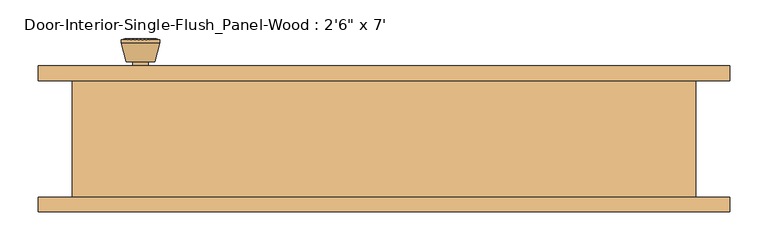
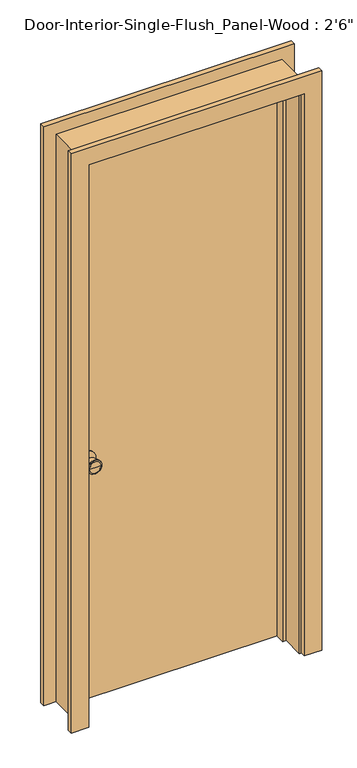
"""IFC4 building model written with IfcOpenShell, lengths in millimetres: door geometry."""

from ifc_helpers import new_model, si_unit, point, frame, frame_2d, origin, origin_with_axes, place, context, project, spatial, polyline, circle_curve, trimmed, segment, composite_curve, outline, extrude, faceted_brep, source, transform, mapped, element, save
from ifc_brep_helpers import plane_surface, cylinder_surface, revolved_surface, advanced_brep


def door_2b62d641(model_context):
    return source(origin(), model_context, "Body", "SolidModel", [
        advanced_brep(
        [(-317.5, 32.1, 914.4), (-307.5, 32.1, 914.4), (-327.5, 32.1, 914.4), (-297.0241324, -16.9, 914.4), (-317.5, -16.9, 914.4), (-337.9758676, -16.9, 914.4), (-292.5, -15.0721319, 914.4), (-342.5, -15.0721319, 914.4), (-292.5, -11.6084537, 914.4), (-342.5, -11.6084537, 914.4), (-298.863764, 13.1, 914.4), (-336.136236, 13.1, 914.4), (-307.5, 13.1, 914.4), (-327.5, 13.1, 914.4)],
        [
            (0, 1),
            (1, 2, circle_curve(frame((-317.5, 32.1, 914.4), z_axis=(0.0, 1.0, 0.0), x_axis=(-1.0, 0.0, 0.0)), 10.0)),
            (2, 0),
            (2, 1, circle_curve(frame((-317.5, 32.1, 914.4), z_axis=(0.0, 1.0, 0.0), x_axis=(-1.0, 0.0, 0.0)), 10.0)),
            (3, 4),
            (4, 5),
            (5, 3, circle_curve(frame((-317.5, -16.9, 914.4), z_axis=(0.0, -1.0, 0.0), x_axis=(-1.0, 0.0, 0.0)), 20.4758676)),
            (3, 5, circle_curve(frame((-317.5, -16.9, 914.4), z_axis=(0.0, -1.0, 0.0), x_axis=(-1.0, 0.0, 0.0)), 20.4758676)),
            (6, 3),
            (5, 7),
            (7, 6, circle_curve(frame((-317.5, -15.0721319, 914.4), z_axis=(0.0, -1.0, 0.0), x_axis=(-1.0, 0.0, 0.0)), 25.0)),
            (6, 7, circle_curve(frame((-317.5, -15.0721319, 914.4), z_axis=(0.0, -1.0, 0.0), x_axis=(-1.0, 0.0, 0.0)), 25.0)),
            (8, 6),
            (7, 9),
            (9, 8, circle_curve(frame((-317.5, -11.6084537, 914.4), z_axis=(0.0, -1.0, 0.0), x_axis=(-1.0, 0.0, 0.0)), 25.0)),
            (8, 9, circle_curve(frame((-317.5, -11.6084537, 914.4), z_axis=(0.0, -1.0, 0.0), x_axis=(-1.0, 0.0, 0.0)), 25.0)),
            (10, 8),
            (9, 11),
            (11, 10, circle_curve(frame((-317.5, 13.1, 914.4), z_axis=(0.0, -1.0, 0.0), x_axis=(-1.0, 0.0, 0.0)), 18.636236)),
            (10, 11, circle_curve(frame((-317.5, 13.1, 914.4), z_axis=(0.0, -1.0, 0.0), x_axis=(-1.0, 0.0, 0.0)), 18.636236)),
            (12, 10),
            (11, 13),
            (13, 12, circle_curve(frame((-317.5, 13.1, 914.4), z_axis=(0.0, -1.0, 0.0), x_axis=(-1.0, 0.0, 0.0)), 10.0)),
            (12, 13, circle_curve(frame((-317.5, 13.1, 914.4), z_axis=(0.0, -1.0, 0.0), x_axis=(-1.0, 0.0, 0.0)), 10.0)),
            (1, 12),
            (13, 2),
        ],
        [
            plane_surface(frame((-317.5, 32.1, 914.4), z_axis=(0.0, 1.0, 0.0), x_axis=(-1.0, 0.0, 0.0))),
            plane_surface(frame((-317.5, -16.9, 914.4), z_axis=(0.0, -1.0, 0.0), x_axis=(-1.0, 0.0, 0.0))),
            revolved_surface(polyline([(-337.9758676, -16.9, 914.4), (-342.5, -15.0721319, 914.4)]), (-317.5, 32.1, 914.4), (0.0, 1.0, 0.0)),
            cylinder_surface(frame((-317.5, 32.1, 914.4), z_axis=(0.0, 1.0, 0.0), x_axis=(-1.0, 0.0, 0.0)), 25.0),
            revolved_surface(polyline([(-342.5, -11.6084537, 914.4), (-336.136236, 13.1, 914.4)]), (-317.5, 32.1, 914.4), (0.0, 1.0, 0.0)),
            plane_surface(frame((-317.5, 13.1, 914.4), z_axis=(0.0, 1.0, 0.0), x_axis=(-1.0, 0.0, 0.0))),
            cylinder_surface(frame((-317.5, 32.1, 914.4), z_axis=(0.0, 1.0, 0.0), x_axis=(-1.0, 0.0, 0.0)), 10.0),
        ],
        [
            (0, [[1, 2, 3]]),
            (0, [[-3, 4, -1]]),
            (1, [[5, 6, 7]]),
            (1, [[-6, -5, 8]]),
            (2, [[9, -7, 10, 11]]),
            (2, [[-10, -8, -9, 12]]),
            (3, [[13, -11, 14, 15]]),
            (3, [[-14, -12, -13, 16]]),
            (4, [[17, -15, 18, 19]]),
            (4, [[-18, -16, -17, 20]]),
            (5, [[21, -19, 22, 23]]),
            (5, [[-22, -20, -21, 24]]),
            (6, [[25, -23, 26, -2]]),
            (6, [[-26, -24, -25, -4]]),
        ],
    ),
        extrude(outline(composite_curve([segment(trimmed(circle_curve(frame_2d((914.4, -317.5)), 30.0), [point((914.4, -347.5))], [point((914.4, -287.5))], False, "CARTESIAN"), True, "CONTINUOUS"), segment(trimmed(circle_curve(frame_2d((914.4, -317.5)), 30.0), [point((914.4, -287.5))], [point((914.4, -347.5))], False, "CARTESIAN"), True, "CONTINUOUS")], self_intersect=False)), frame((0.0, 32.1, 0.0), z_axis=(0.0, 1.0, 0.0), x_axis=(0.0, 0.0, 1.0)), (0.0, 0.0, 1.0), 6.0),
        advanced_brep(
        [(-317.5, 79.025, 914.4), (-327.5, 79.025, 914.4), (-307.5, 79.025, 914.4), (-297.0241324, 128.025, 914.4), (-337.9758676, 128.025, 914.4), (-317.5, 128.025, 914.4), (-292.5, 126.1971319, 914.4), (-342.5, 126.1971319, 914.4), (-292.5, 122.7334537, 914.4), (-342.5, 122.7334537, 914.4), (-298.863764, 98.025, 914.4), (-336.136236, 98.025, 914.4), (-307.5, 98.025, 914.4), (-327.5, 98.025, 914.4)],
        [
            (0, 1),
            (1, 2, circle_curve(frame((-317.5, 79.025, 914.4), z_axis=(0.0, -1.0, 0.0), x_axis=(-1.0, 0.0, 0.0)), 10.0)),
            (2, 0),
            (2, 1, circle_curve(frame((-317.5, 79.025, 914.4), z_axis=(0.0, -1.0, 0.0), x_axis=(-1.0, 0.0, 0.0)), 10.0)),
            (3, 4, circle_curve(frame((-317.5, 128.025, 914.4), z_axis=(0.0, 1.0, 0.0), x_axis=(-1.0, 0.0, 0.0)), 20.4758676)),
            (4, 5),
            (5, 3),
            (4, 3, circle_curve(frame((-317.5, 128.025, 914.4), z_axis=(0.0, 1.0, 0.0), x_axis=(-1.0, 0.0, 0.0)), 20.4758676)),
            (6, 7, circle_curve(frame((-317.5, 126.1971319, 914.4), z_axis=(0.0, 1.0, 0.0), x_axis=(-1.0, 0.0, 0.0)), 25.0)),
            (7, 4),
            (3, 6),
            (7, 6, circle_curve(frame((-317.5, 126.1971319, 914.4), z_axis=(0.0, 1.0, 0.0), x_axis=(-1.0, 0.0, 0.0)), 25.0)),
            (8, 9, circle_curve(frame((-317.5, 122.7334537, 914.4), z_axis=(0.0, 1.0, 0.0), x_axis=(-1.0, 0.0, 0.0)), 25.0)),
            (9, 7),
            (6, 8),
            (9, 8, circle_curve(frame((-317.5, 122.7334537, 914.4), z_axis=(0.0, 1.0, 0.0), x_axis=(-1.0, 0.0, 0.0)), 25.0)),
            (10, 11, circle_curve(frame((-317.5, 98.025, 914.4), z_axis=(0.0, 1.0, 0.0), x_axis=(-1.0, 0.0, 0.0)), 18.636236)),
            (11, 9),
            (8, 10),
            (11, 10, circle_curve(frame((-317.5, 98.025, 914.4), z_axis=(0.0, 1.0, 0.0), x_axis=(-1.0, 0.0, 0.0)), 18.636236)),
            (12, 13, circle_curve(frame((-317.5, 98.025, 914.4), z_axis=(0.0, 1.0, 0.0), x_axis=(-1.0, 0.0, 0.0)), 10.0)),
            (13, 11),
            (10, 12),
            (13, 12, circle_curve(frame((-317.5, 98.025, 914.4), z_axis=(0.0, 1.0, 0.0), x_axis=(-1.0, 0.0, 0.0)), 10.0)),
            (1, 13),
            (12, 2),
        ],
        [
            plane_surface(frame((-317.5, 79.025, 914.4), z_axis=(0.0, -1.0, 0.0), x_axis=(-1.0, 0.0, 0.0))),
            plane_surface(frame((-317.5, 128.025, 914.4), z_axis=(0.0, 1.0, 0.0), x_axis=(-1.0, 0.0, 0.0))),
            revolved_surface(polyline([(-337.9758676, 128.025, 914.4), (-342.5, 126.1971319, 914.4)]), (-317.5, 79.025, 914.4), (0.0, -1.0, 0.0)),
            cylinder_surface(frame((-317.5, 79.025, 914.4), z_axis=(0.0, -1.0, 0.0), x_axis=(-1.0, 0.0, 0.0)), 25.0),
            revolved_surface(polyline([(-342.5, 122.7334537, 914.4), (-336.136236, 98.025, 914.4)]), (-317.5, 79.025, 914.4), (0.0, -1.0, 0.0)),
            plane_surface(frame((-317.5, 98.025, 914.4), z_axis=(0.0, -1.0, 0.0), x_axis=(-1.0, 0.0, 0.0))),
            cylinder_surface(frame((-317.5, 79.025, 914.4), z_axis=(0.0, -1.0, 0.0), x_axis=(-1.0, 0.0, 0.0)), 10.0),
        ],
        [
            (0, [[1, 2, 3]]),
            (0, [[-3, 4, -1]]),
            (1, [[5, 6, 7]]),
            (1, [[8, -7, -6]]),
            (2, [[9, 10, -5, 11]]),
            (2, [[12, -11, -8, -10]]),
            (3, [[13, 14, -9, 15]]),
            (3, [[16, -15, -12, -14]]),
            (4, [[17, 18, -13, 19]]),
            (4, [[20, -19, -16, -18]]),
            (5, [[21, 22, -17, 23]]),
            (5, [[24, -23, -20, -22]]),
            (6, [[-2, 25, -21, 26]]),
            (6, [[-4, -26, -24, -25]]),
        ],
    ),
        extrude(outline(composite_curve([segment(trimmed(circle_curve(frame_2d((914.4, -317.5)), 30.0), [point((914.4, -347.5))], [point((914.4, -287.5))], False, "CARTESIAN"), True, "CONTINUOUS"), segment(trimmed(circle_curve(frame_2d((914.4, -317.5)), 30.0), [point((914.4, -287.5))], [point((914.4, -347.5))], False, "CARTESIAN"), True, "CONTINUOUS")], self_intersect=False)), frame((0.0, 73.025, 0.0), z_axis=(0.0, 1.0, 0.0), x_axis=(0.0, 0.0, 1.0)), (0.0, 0.0, 1.0), 6.0),
        faceted_brep([(406.4, 73.025, 0.0), (406.4, -79.375, 0.0), (381.0, -79.375, 0.0), (381.0, 3.175, 0.0), (368.3, 3.175, 0.0), (368.3, 38.1, 0.0), (381.0, 38.1, 0.0), (381.0, 73.025, 0.0), (406.4, 73.025, 2159.0), (406.4, -79.375, 2159.0), (-406.4, -79.375, 2159.0), (-406.4, -79.375, 0.0), (-381.0, -79.375, 0.0), (-381.0, -79.375, 2133.6), (381.0, -79.375, 2133.6), (381.0, 3.175, 2133.6), (-381.0, 3.175, 2133.6), (-381.0, 3.175, 0.0), (-368.3, 3.175, 0.0), (-368.3, 3.175, 2120.9), (368.3, 3.175, 2120.9), (368.3, 38.1, 2120.9), (-368.3, 38.1, 2120.9), (-368.3, 38.1, 0.0), (-381.0, 38.1, 0.0), (-381.0, 38.1, 2133.6), (381.0, 38.1, 2133.6), (381.0, 73.025, 2133.6), (-381.0, 73.025, 2133.6), (-381.0, 73.025, 0.0), (-406.4, 73.025, 0.0), (-406.4, 73.025, 2159.0)], [[[0, 1, 2, 3, 4, 5, 6, 7]], [[1, 0, 8, 9]], [[2, 1, 9, 10, 11, 12, 13, 14]], [[3, 2, 14, 15]], [[4, 3, 15, 16, 17, 18, 19, 20]], [[5, 4, 20, 21]], [[6, 5, 21, 22, 23, 24, 25, 26]], [[7, 6, 26, 27]], [[0, 7, 27, 28, 29, 30, 31, 8]], [[9, 8, 31, 10]], [[15, 14, 13, 16]], [[21, 20, 19, 22]], [[27, 26, 25, 28]], [[30, 29, 24, 23, 18, 17, 12, 11]], [[10, 31, 30, 11]], [[16, 13, 12, 17]], [[22, 19, 18, 23]], [[28, 25, 24, 29]]]),
        extrude(outline(polyline([(381.0, 38.1), (-381.0, 38.1), (-381.0, 73.025), (381.0, 73.025), (381.0, 38.1)])), origin_with_axes(), (0.0, 0.0, 1.0), 2133.6),
        extrude(outline(polyline([(0.0, 387.35), (0.0, 450.85), (2203.45, 450.85), (2203.45, -450.85), (0.0, -450.85), (0.0, -387.35), (2139.95, -387.35), (2139.95, 387.35), (0.0, 387.35)])), frame((0.0, 73.025, 0.0), z_axis=(0.0, 1.0, 0.0), x_axis=(0.0, 0.0, 1.0)), (0.0, 0.0, 1.0), 19.05),
        extrude(outline(polyline([(0.0, 387.35), (0.0, 450.85), (2203.45, 450.85), (2203.45, -450.85), (0.0, -450.85), (0.0, -387.35), (2139.95, -387.35), (2139.95, 387.35), (0.0, 387.35)])), frame((0.0, -98.425, 0.0), z_axis=(0.0, 1.0, 0.0), x_axis=(0.0, 0.0, 1.0)), (0.0, 0.0, 1.0), 19.05),
    ])


if __name__ == "__main__":
    model = new_model("IFC4")
    model_context = context("Model", 3, world=origin())
    ifc_project = project(units=[si_unit("LENGTHUNIT", "METRE", prefix="MILLI")], contexts=[model_context])
    site = spatial("IfcSite", under=ifc_project)
    building = spatial("IfcBuilding", under=site)
    placement = place(None, origin())
    door_shape = door_2b62d641(model_context)
    element("IfcDoor", 1, ObjectType="Door-Interior-Single-Flush_Panel-Wood : 2'6\" x 7'", at=placement, inside=building, context=model_context, shape_type="MappedRepresentation", body=[
        mapped(door_shape, transform((0.0, 0.0, 0.0), x_axis=(1.0, 0.0, 0.0), y_axis=(0.0, 1.0, 0.0), z_axis=(0.0, 0.0, 1.0))),
    ])
    save(model, "model.ifc")

# Revit data of these elements
# Type "Door-Interior-Single-Flush_Panel-Wood : 2'6\" x 7'"
#   Type Mark = "13"
#   Assembly Code = "C1020300"
#   Analytic Construction = "Wooden"
#   Thickness = 0' - 1 3/8"
#   Thermal Resistance (R) = 2.5876 (h·ft²·°F)/BTU
#   Swing Angle [instance default] = 90.00°
#   Rough Width = 2' - 8"
#   Rough Height = 7' - 1"
#   Height = 7' - 0"
#   Width = 2' - 6"
#   Heat Transfer Coefficient (U) = 0.3865 BTU/(h·ft²·°F)
#   Trim Material = Cherry
#   Panel Material = Cherry
#   Frame Material = Cherry
#   Door Handle Material = Aluminum
#   Visual Light Transmittance = 0
#   Solar Heat Gain Coefficient = 0
#   Wall Closure = (empty or 0)
#   Function = (empty or 0)
# Element 1 (IfcDoor, "Door-Interior-Single-Flush_Panel-Wood : 2'6\" x 7'")
#   Materials on its faces: "Cherry", "Aluminum"
# Materials
#   "Cherry": class "Wood", colour RGB 226 177 128, transparency 0, Description = "Prunus Serotina", Cost = 0
#   "Aluminum": class "Metal", colour RGB 247 247 247, transparency 0, Description = "Aluminum 6061", Cost = 0
